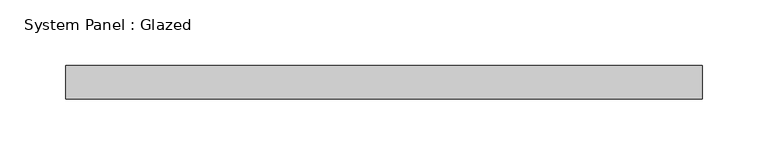
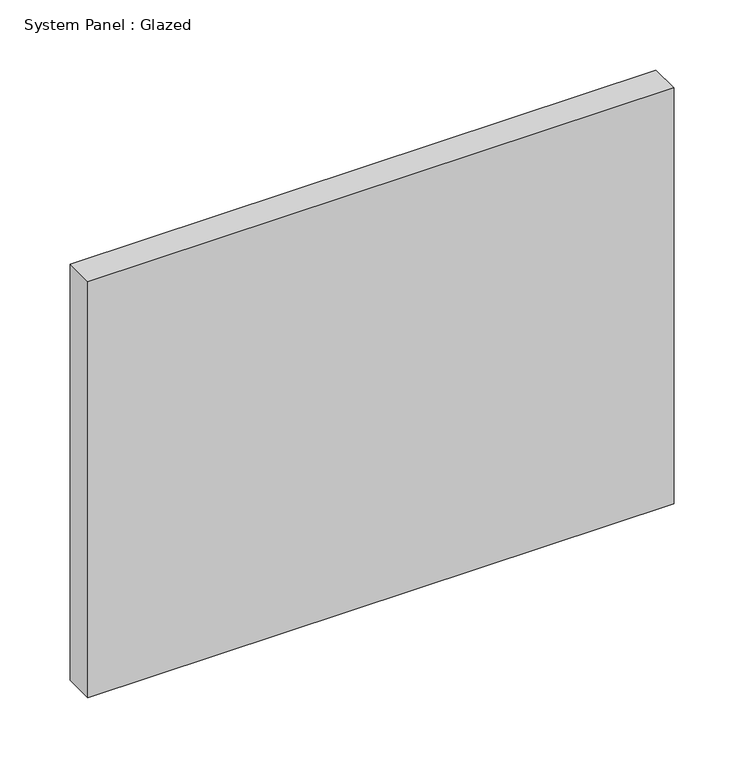
"""IFC4 building model written with IfcOpenShell, lengths in millimetres: plate geometry, System Panel : Glazed."""

from ifc_helpers import new_model, si_unit, origin, origin_with_axes, place, context, project, spatial, polyline, outline, extrude, source, transform, mapped, element, save


def system_panel_glazed_6fd79a86(model_context):
    return source(origin(), model_context, "Body", "SweptSolid", [
        extrude(outline(polyline([(241.3, 19.05), (-241.3, 19.05), (-241.3, 44.45), (241.3, 44.45), (241.3, 19.05)])), origin_with_axes(), (0.0, 0.0, 1.0), 361.95),
    ])


if __name__ == "__main__":
    model = new_model("IFC4")
    model_context = context("Model", 3, world=origin())
    ifc_project = project(units=[si_unit("LENGTHUNIT", "METRE", prefix="MILLI")], contexts=[model_context])
    site = spatial("IfcSite", under=ifc_project)
    building = spatial("IfcBuilding", under=site)
    placement = place(None, origin())
    system_panel_glazed_shape = system_panel_glazed_6fd79a86(model_context)
    element("IfcPlate", 1, ObjectType="System Panel : Glazed", at=placement, inside=building, context=model_context, shape_type="MappedRepresentation", body=[
        mapped(system_panel_glazed_shape, transform((0.0, 0.0, 0.0), x_axis=(1.0, 0.0, 0.0), y_axis=(0.0, 1.0, 0.0), z_axis=(0.0, 0.0, 1.0))),
    ])
    save(model, "model.ifc")

# Revit data of these elements
# Type "System Panel : Glazed"
#   Construction Type Id = "GSP4R"
#   Analytic Construction = "1/8 in Pilkington single glazing"
#   Visual Light Transmittance = 0.9
#   Solar Heat Gain Coefficient = 0.86
#   Heat Transfer Coefficient (U) = 1.18115 BTU/(h·ft²·°F)
#   Define Thermal Properties by = 1
# Element 1 (IfcPlate, "System Panel : Glazed")
#   Materials on its faces: "Glass"
# Materials
#   "Glass": class "Glass", colour RGB 0 128 192, transparency 0.75, Description = "Soda Lime Glass", Cost = 0
